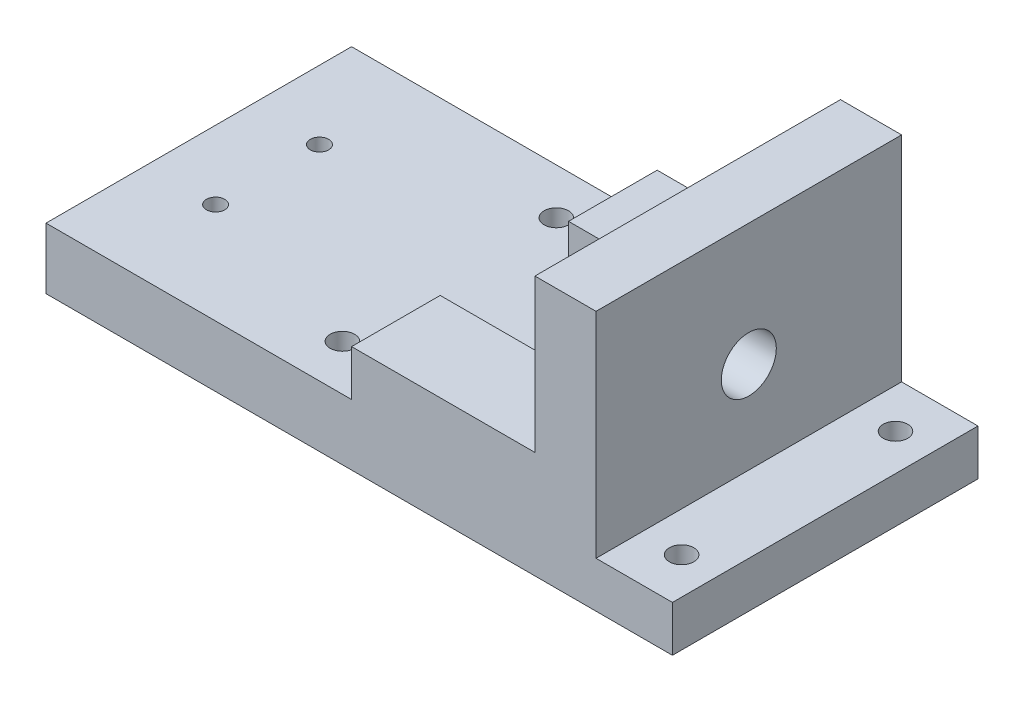
SolidWorks part; units mm, degrees
material "Plain Carbon Steel"
ref_plane "Front Plane" through (0, 0, 0) normal (0, 0, 1) x (1, 0, 0)
ref_plane "Top Plane" through (0, 0, 0) normal (0, 1, 0) x (1, 0, 0)
ref_plane "Right Plane" through (0, 0, 0) normal (1, 0, 0) x (0, 0, -1)
sketch "Bracket Profile Sketch" plane through (0, 0, 0) normal (0, 0, 1) x (1, 0, 0)
  line L0 (0, 0) -> (-102.5, 0)
  line L1 (-102.5, 0) -> (-102.5, 20)
  line L2 (-102.5, 20) -> (-2.5, 20)
  line L3 (-2.5, 20) -> (-2.5, 35)
  line L4 (-2.5, 35) -> (57.5, 35)
  line L5 (57.5, 35) -> (57.5, 85)
  line L6 (57.5, 85) -> (77.5, 85)
  line L7 (77.5, 85) -> (77.5, 15)
  line L8 (77.5, 15) -> (102.5, 15)
  line L9 (102.5, 15) -> (102.5, 0)
  line L10 (102.5, 0) -> (0, 0)
  dimension "D1" = 205
  dimension "D2" = 20
  dimension "D3" = 15
  dimension "D4" = 60
  dimension "D5" = 50
  dimension "D6" = 20
  dimension "D7" = 100
  dimension "D8" = 15
  dimension "D9" = 102.5
extrude "Bracket Body" add sketch "Bracket Profile Sketch" along normal mid plane 100
sketch "Base Holes Ø8 Set A Sketch" plane through (0, 15, 0) normal (0, 1, 0) x (1, 0, 0)
  line L0 (102.5, -50) -> (102.5, 50) construction
  line L1 (102.5, 50) -> (77.5, 50) construction
  line L2 (0, 0) -> (40.093, 0) construction
  circle A0 centre (90.5, 35) radius 4
  circle A2 centre (90.5, -35) radius 4
  dimension "D1" = 8
  dimension "D2" = 12
  dimension "D3" = 15
extrude "Base Holes Ø8 Set A" cut sketch "Base Holes Ø8 Set A Sketch" against normal blind 100
sketch "Step Notch Sketch" plane through (0, 35, 0) normal (0, 1, 0) x (1, 0, 0)
  line L0 (57.5, -21) -> (57.5, 21)
  line L2 (57.5, -50) -> (57.5, 50) construction
  line L3 (57.5, 21) -> (-2.5, 21)
  line L4 (-2.5, -50) -> (-2.5, 50) construction
  line L5 (-2.5, 21) -> (-2.5, -21)
  line L6 (-2.5, -50) -> (-2.5, 50) construction
  line L7 (-2.5, -21) -> (57.5, -21)
  point P3 (57.5, 0)
  dimension "D1" = 42
  dimension "D2" = 21
  dimension "D3" = 60
  dimension "D4" = 21
extrude "Step Notch" cut sketch "Step Notch Sketch" against normal up to surface (15 mm away) up to face at (-52.5, 20, 0)
sketch "Web Bore Ø18 Sketch" plane through (77.5, 0, 0) normal (1, 0, 0) x (0, 0, -1)
  line L0 (-50, 0) -> (50, 0) construction
  circle A0 centre (0, 45) radius 9
  dimension "D1" = 18
  dimension "D2" = 45
extrude "Web Bore Ø18" cut sketch "Web Bore Ø18 Sketch" along direction (1, 0, 0) on the side against the normal blind 100
sketch "Base Holes Ø8 Set B Sketch" plane through (0, 20, 0) normal (0, 1, 0) x (1, 0, 0)
  line L0 (-102.5, -50) -> (-102.5, 50) construction
  line L1 (0, 0) -> (44.3497, 0) construction
  circle A0 centre (-20.5, -35) radius 4
  circle A1 centre (-20.5, 35) radius 4
  dimension "D1" = 8
  dimension "D2" = 82
  dimension "D3" = 35
extrude "Base Holes Ø8 Set B" cut sketch "Base Holes Ø8 Set B Sketch" against normal blind 100
sketch "Base Holes Ø6 Sketch" plane through (0, 20, 0) normal (0, 1, 0) x (1, 0, 0)
  line L0 (-102.5, -50) -> (-102.5, 50) construction
  line L1 (0, 0) -> (47.9166, 0) construction
  circle A0 centre (-80, -17) radius 3
  circle A1 centre (-80, 17) radius 3
  dimension "D1" = 6
  dimension "D2" = 22.5
  dimension "D3" = 17
extrude "Base Holes Ø6" cut sketch "Base Holes Ø6 Sketch" against normal blind 100
